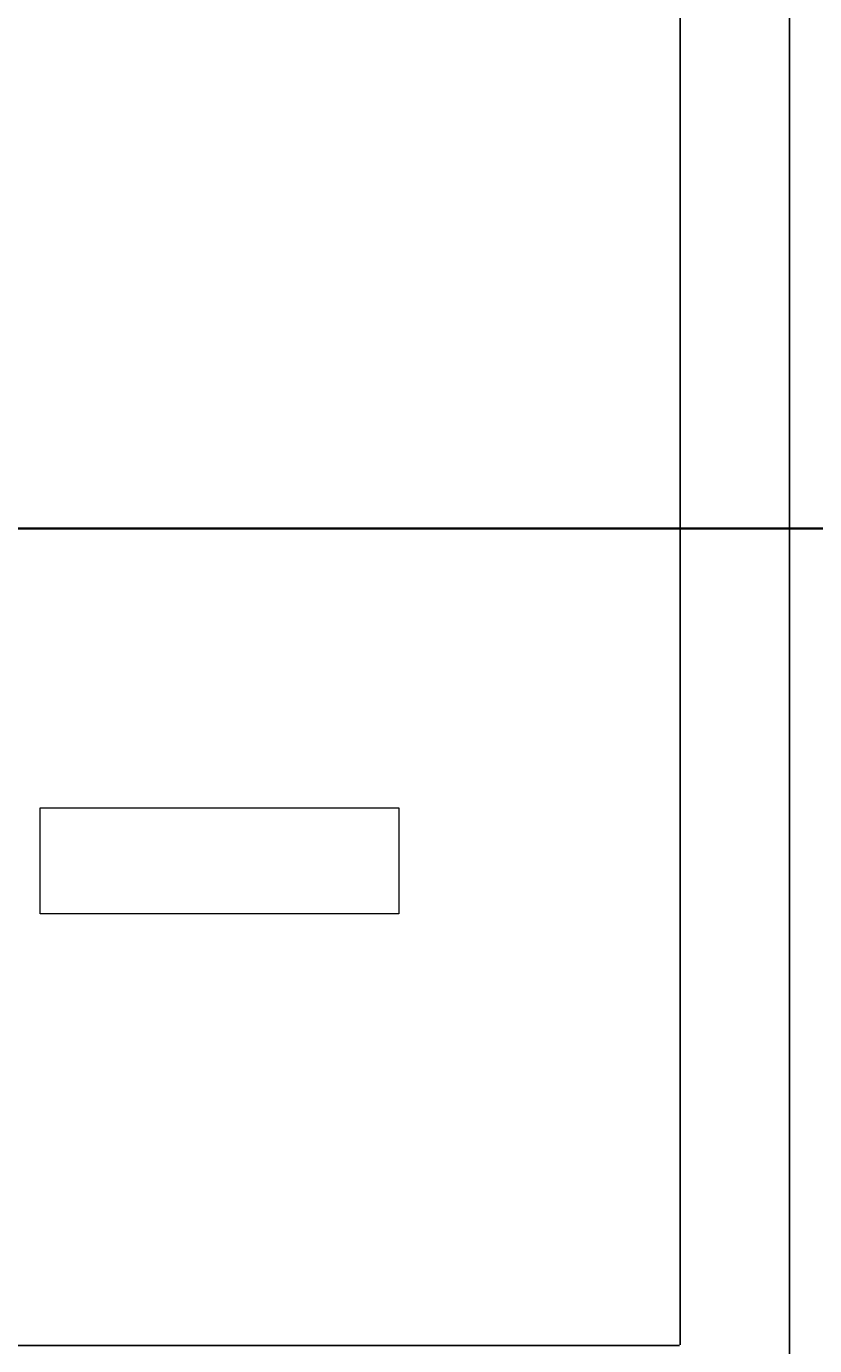
# Model space of a CAD drawing. Units: inches. Extents: x -26 to 776, y -22 to 650.
# Tile 27 of 62: x 25 to 94, y 420 to 535. Entities that reach past the tile are written whole.
import ezdxf

# ---------------------------------------------------------------- set-up
doc = ezdxf.new("R2010")
doc.units = ezdxf.units.IN
doc.header["$MEASUREMENT"] = 0
for name, color, linetype, lineweight in [('A-ANNO-DIMS', 2, 'Continuous', 18), ('A-WALL', 7, 'Continuous', 35), ('A-WALL-TRIM', 7, 'Continuous', 18)]:
    doc.layers.add(name, color=color, linetype=linetype, lineweight=lineweight)
doc.styles.get("Standard").update_dxf_attribs({"font": 'arial.ttf'})
doc.dimstyles.get("Standard").update_dxf_attribs({"dimtxt": 0.5625, "dimasz": 0.18, "dimexe": 0.18, "dimexo": 0.0625, "dimgap": 0.09, "dimtad": 0, "dimtih": 1, "dimtoh": 1, "dimdec": 4, "dimzin": 0, "dimdsep": 46, "dimlunit": 4, "dimtxsty": 'Standard', "dimcen": 0.09, "dimadec": 0, "dimazin": 0, "dimtfac": 1, "dimtdec": 4, "dimtofl": 0, "dimtmove": 0, "dimatfit": 3, "dimfxl": 1, "dimtolj": 1, "dimtzin": 0, "dimarcsym": 0})

# ---------------------------------------------------------------- blocks, each defined once
blk = doc.blocks.new('*D14')
at = {"layer": 'A-ANNO-DIMS', "color": 0, "lineweight": -2, "transparency": 16777216}
for p, q in [((191.62, 613.27), (-25.48, 613.27)), ((-25.3, 613.09), (-25.3, 314.75)), ((-25.3, 15.66), (-25.3, 314)), ((11.04, 15.48), (-25.48, 15.48))]:
    blk.add_line(p, q, dxfattribs=at)
at = {"layer": 'A-ANNO-DIMS', "color": 0, "transparency": 16777216}
for points in [[(-25.33, 613.09), (-25.27, 613.09), (-25.3, 613.27)], [(-25.33, 15.66), (-25.27, 15.66), (-25.3, 15.48)]]:
    blk.add_solid(points, dxfattribs=at)
at = {"layer": 'Defpoints', "color": 0, "transparency": 16777216}
for p in [(-25.3, 613.27), (191.68, 613.27), (11.11, 15.48)]:
    blk.add_point(p, dxfattribs=at)
at = {"layer": 'A-ANNO-DIMS', "color": 0, "transparency": 16777216, "insert": (-25.3, 314.38), "char_height": 0.562, "attachment_point": 5}
blk.add_mtext('\\A1;597.8', dxfattribs=at)
blk = doc.blocks.new('*D15')
at = {"layer": 'A-ANNO-DIMS', "color": 0, "lineweight": -2, "transparency": 16777216}
for p, q in [((11.11, 491.49), (11.11, 649.86)), ((11.29, 649.68), (120.22, 649.68)), ((231.24, 649.68), (122.31, 649.68)), ((231.42, 491.49), (231.42, 649.86))]:
    blk.add_line(p, q, dxfattribs=at)
at = {"layer": 'A-ANNO-DIMS', "color": 0, "transparency": 16777216}
for points in [[(11.29, 649.71), (11.29, 649.65), (11.11, 649.68)], [(231.24, 649.71), (231.24, 649.65), (231.42, 649.68)]]:
    blk.add_solid(points, dxfattribs=at)
at = {"layer": 'Defpoints', "color": 0, "transparency": 16777216}
for p in [(231.42, 649.68), (11.11, 491.43), (231.42, 491.43)]:
    blk.add_point(p, dxfattribs=at)
at = {"layer": 'A-ANNO-DIMS', "color": 0, "transparency": 16777216, "insert": (121.27, 649.68), "char_height": 0.562, "attachment_point": 5}
blk.add_mtext('\\A1;220.3', dxfattribs=at)
blk = doc.blocks.new('*D17')
at = {"layer": 'A-ANNO-DIMS', "color": 0, "lineweight": -2, "transparency": 16777216}
for p, q in [((11.11, 491.49), (11.11, 649.86)), ((11.29, 649.68), (100.16, 649.68)), ((191.5, 649.68), (102.62, 649.68)), ((191.68, 613.33), (191.68, 649.86))]:
    blk.add_line(p, q, dxfattribs=at)
at = {"layer": 'A-ANNO-DIMS', "color": 0, "transparency": 16777216}
for points in [[(11.29, 649.71), (11.29, 649.65), (11.11, 649.68)], [(191.5, 649.71), (191.5, 649.65), (191.68, 649.68)]]:
    blk.add_solid(points, dxfattribs=at)
at = {"layer": 'Defpoints', "color": 0, "transparency": 16777216}
for p in [(191.68, 649.68), (191.68, 613.27), (11.11, 491.43)]:
    blk.add_point(p, dxfattribs=at)
at = {"layer": 'A-ANNO-DIMS', "color": 0, "transparency": 16777216, "insert": (101.39, 649.68), "char_height": 0.562, "attachment_point": 5}
blk.add_mtext('\\A1;180.57', dxfattribs=at)
blk = doc.blocks.new('*D19')
at = {"layer": 'A-ANNO-DIMS', "color": 0, "lineweight": -2, "transparency": 16777216}
for p, q in [((191.62, 613.27), (-25.48, 613.27)), ((-25.3, 613.09), (-25.3, 552.73)), ((-25.3, 491.61), (-25.3, 551.97)), ((191.62, 491.43), (-25.48, 491.43))]:
    blk.add_line(p, q, dxfattribs=at)
at = {"layer": 'A-ANNO-DIMS', "color": 0, "transparency": 16777216}
for points in [[(-25.33, 613.09), (-25.27, 613.09), (-25.3, 613.27)], [(-25.33, 491.61), (-25.27, 491.61), (-25.3, 491.43)]]:
    blk.add_solid(points, dxfattribs=at)
at = {"layer": 'Defpoints', "color": 0, "transparency": 16777216}
for p in [(-25.3, 613.27), (191.68, 613.27), (191.68, 491.43)]:
    blk.add_point(p, dxfattribs=at)
at = {"layer": 'A-ANNO-DIMS', "color": 0, "transparency": 16777216, "insert": (-25.3, 552.35), "char_height": 0.562, "attachment_point": 5}
blk.add_mtext('\\A1;121.84', dxfattribs=at)
blk = doc.blocks.new('*D22')
at = {"layer": 'A-ANNO-DIMS', "color": 0, "lineweight": -2, "transparency": 16777216}
for p, q in [((22.89, 15.33), (22.89, 649.86)), ((23.07, 649.68), (119.19, 649.68)), ((217.77, 649.68), (121.65, 649.68)), ((217.95, 15.54), (217.95, 649.86))]:
    blk.add_line(p, q, dxfattribs=at)
at = {"layer": 'A-ANNO-DIMS', "color": 0, "transparency": 16777216}
for points in [[(23.07, 649.71), (23.07, 649.65), (22.89, 649.68)], [(217.77, 649.71), (217.77, 649.65), (217.95, 649.68)]]:
    blk.add_solid(points, dxfattribs=at)
at = {"layer": 'Defpoints', "color": 0, "transparency": 16777216}
for p in [(217.95, 649.68), (22.89, 15.27), (217.95, 15.48)]:
    blk.add_point(p, dxfattribs=at)
at = {"layer": 'A-ANNO-DIMS', "color": 0, "transparency": 16777216, "insert": (120.42, 649.68), "char_height": 0.562, "attachment_point": 5}
blk.add_mtext('\\A1;195.06', dxfattribs=at)
blk = doc.blocks.new('*D25')
at = {"layer": 'A-ANNO-DIMS', "color": 0, "lineweight": -2, "transparency": 16777216}
for p, q in [((11.11, 221.7), (11.11, 649.86)), ((11.29, 649.68), (50.34, 649.68)), ((91.46, 649.68), (52.41, 649.68)), ((91.64, 271.37), (91.64, 649.86))]:
    blk.add_line(p, q, dxfattribs=at)
at = {"layer": 'A-ANNO-DIMS', "color": 0, "transparency": 16777216}
for points in [[(11.29, 649.71), (11.29, 649.65), (11.11, 649.68)], [(91.46, 649.71), (91.46, 649.65), (91.64, 649.68)]]:
    blk.add_solid(points, dxfattribs=at)
at = {"layer": 'Defpoints', "color": 0, "transparency": 16777216}
for p in [(91.64, 649.68), (91.64, 271.31), (11.11, 221.64)]:
    blk.add_point(p, dxfattribs=at)
at = {"layer": 'A-ANNO-DIMS', "color": 0, "transparency": 16777216, "insert": (51.38, 649.68), "char_height": 0.562, "attachment_point": 5}
blk.add_mtext('\\A1;80.54', dxfattribs=at)
blk = doc.blocks.new('*D35')
at = {"layer": 'A-ANNO-DIMS', "color": 0, "lineweight": -2, "transparency": 16777216}
for p, q in [((82.13, 420.34), (82.13, 649.86)), ((82.31, 649.68), (144.38, 649.68)), ((208.91, 649.68), (146.84, 649.68)), ((209.09, 420.34), (209.09, 649.86))]:
    blk.add_line(p, q, dxfattribs=at)
at = {"layer": 'A-ANNO-DIMS', "color": 0, "transparency": 16777216}
for points in [[(82.31, 649.71), (82.31, 649.65), (82.13, 649.68)], [(208.91, 649.71), (208.91, 649.65), (209.09, 649.68)]]:
    blk.add_solid(points, dxfattribs=at)
at = {"layer": 'Defpoints', "color": 0, "transparency": 16777216}
for p in [(209.09, 649.68), (82.13, 420.28), (209.09, 420.28)]:
    blk.add_point(p, dxfattribs=at)
at = {"layer": 'A-ANNO-DIMS', "color": 0, "transparency": 16777216, "insert": (145.61, 649.68), "char_height": 0.562, "attachment_point": 5}
blk.add_mtext('\\A1;126.96', dxfattribs=at)
blk = doc.blocks.new('*D36')
at = {"layer": 'A-ANNO-DIMS', "color": 0, "lineweight": -2, "transparency": 16777216}
for p, q in [((82.07, 420.28), (-25.48, 420.28)), ((-25.3, 420.1), (-25.3, 290.26)), ((-25.3, 159.66), (-25.3, 289.5)), ((82.07, 159.48), (-25.48, 159.48))]:
    blk.add_line(p, q, dxfattribs=at)
at = {"layer": 'A-ANNO-DIMS', "color": 0, "transparency": 16777216}
for points in [[(-25.33, 420.1), (-25.27, 420.1), (-25.3, 420.28)], [(-25.33, 159.66), (-25.27, 159.66), (-25.3, 159.48)]]:
    blk.add_solid(points, dxfattribs=at)
at = {"layer": 'Defpoints', "color": 0, "transparency": 16777216}
for p in [(-25.3, 420.28), (82.13, 420.28), (82.13, 159.48)]:
    blk.add_point(p, dxfattribs=at)
at = {"layer": 'A-ANNO-DIMS', "color": 0, "transparency": 16777216, "insert": (-25.3, 289.88), "char_height": 0.562, "attachment_point": 5}
blk.add_mtext('\\A1;260.8', dxfattribs=at)

msp = doc.modelspace()

# ---------------------------------------------------------------- linework, layer by layer
at = {"layer": 'A-WALL'}
msp.add_line((11.1074, 491.4269), (231.4249, 491.4269), dxfattribs=at)
at = {"layer": 'A-WALL-TRIM'}
msp.add_lwpolyline([(26.3772, 467.0974), (57.6098, 467.0974), (57.6098, 457.877), (26.3772, 457.877)], close=True, dxfattribs=at)

# ---------------------------------------------------------------- dimensions: what is measured, and where the dimension line sits
at = {"layer": 'A-ANNO-DIMS'}
for base, p1, p2, override, picture, middle in [((231.4249, 649.6763), (11.1074, 491.4269), (231.4249, 491.4269), {"dimdec": 1, "dimlfac": 1, "dimrnd": 0, "dimzin": 0, "dimdsep": 46, "dimlunit": 2}, '*D15', (121.2661, 649.6763)), ((191.6782, 649.6763), (11.1074, 491.4269), (191.6782, 613.2713), {"dimdec": 2, "dimlfac": 1, "dimrnd": 0, "dimzin": 0, "dimdsep": 46, "dimlunit": 2}, '*D17', (101.3928, 649.6763)), ((91.6448, 649.6763), (11.1074, 221.6413), (91.6448, 271.3091), {"dimdec": 2, "dimlfac": 1, "dimrnd": 0, "dimzin": 0, "dimdsep": 46, "dimlunit": 2}, '*D25', (51.3761, 649.6763)), ((217.9529, 649.6763), (22.8891, 15.2701), (217.9529, 15.4824), {"dimdec": 2, "dimlfac": 1, "dimrnd": 0, "dimzin": 0, "dimdsep": 46, "dimlunit": 2}, '*D22', (120.421, 649.6763)), ((209.091, 649.6763), (82.134, 420.2783), (209.091, 420.2783), {"dimdec": 2, "dimlfac": 1, "dimrnd": 0, "dimzin": 0, "dimdsep": 46, "dimlunit": 2}, '*D35', (145.6125, 649.6763))]:
    dim = msp.add_linear_dim(base=base, p1=p1, p2=p2, dimstyle='Standard', override=override, dxfattribs=at)
    dim.commit()
    dim.dimension.update_dxf_attribs({"geometry": picture, "text_midpoint": middle})
for base, p1, p2, override, picture, middle in [((-25.2976, 613.2713), (191.6782, 491.4269), (191.6782, 613.2713), {"dimdec": 2, "dimlfac": 1, "dimrnd": 0, "dimzin": 0, "dimdsep": 46, "dimlunit": 2}, '*D19', (-25.2976, 552.3491)), ((-25.2976, 613.2713), (11.1074, 15.4824), (191.6782, 613.2713), {"dimdec": 1, "dimlfac": 1, "dimrnd": 0, "dimzin": 0, "dimdsep": 46, "dimlunit": 2}, '*D14', (-25.2976, 314.3769)), ((-25.2976, 420.2783), (82.134, 159.4824), (82.134, 420.2783), {"dimdec": 1, "dimlfac": 1, "dimrnd": 0, "dimzin": 0, "dimdsep": 46, "dimlunit": 2}, '*D36', (-25.2976, 289.8803))]:
    dim = msp.add_linear_dim(base=base, p1=p1, p2=p2, angle=90, dimstyle='Standard', override=override, dxfattribs=at)
    dim.commit()
    dim.dimension.update_dxf_attribs({"geometry": picture, "text_midpoint": middle})

doc.saveas('drawing.dxf')
